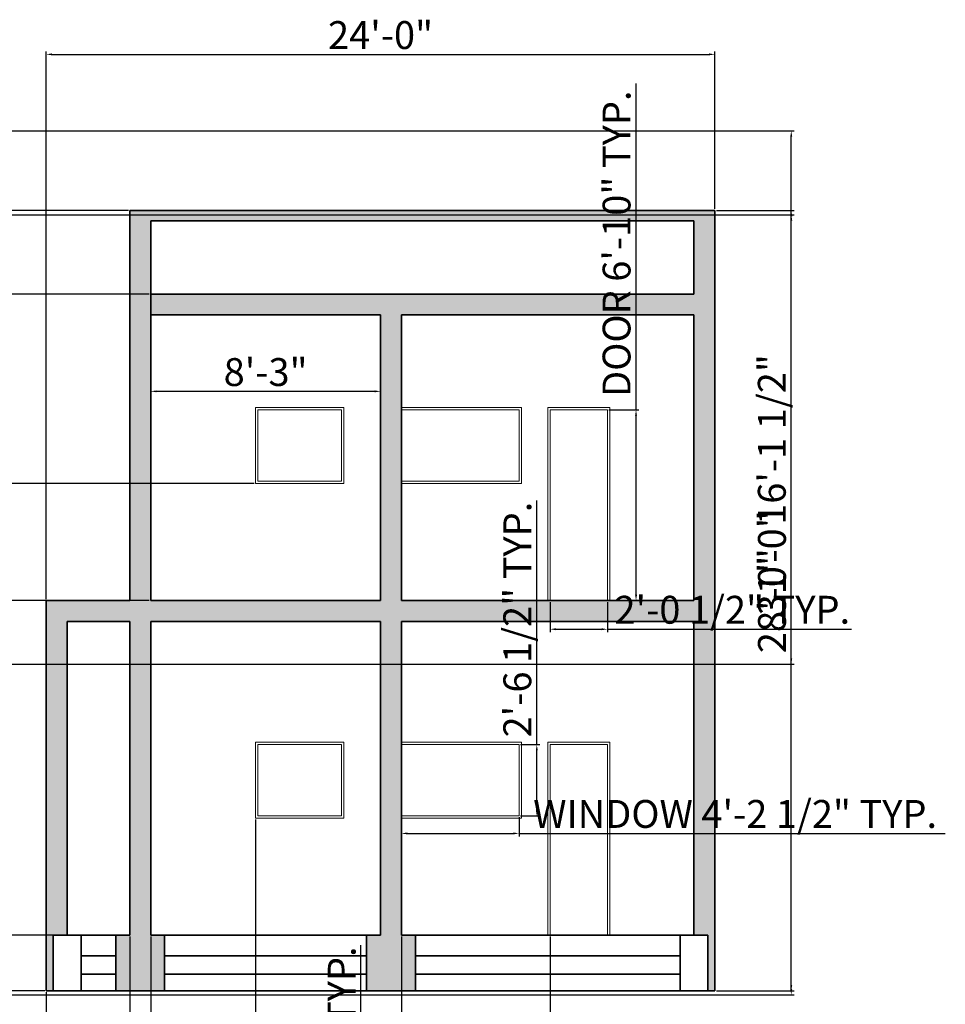
# Model space of a CAD drawing. Units: inches. Extents: x 2693 to 3501, y 1190 to 2292.
# Tile 4 of 4: x 3102 to 3501, y 1858 to 2282. Entities that reach past the tile are written whole.
import ezdxf

# ---------------------------------------------------------------- set-up
doc = ezdxf.new("R2010")
doc.units = ezdxf.units.IN
for name, color, linetype, lineweight in [('A-ANNO-DIMS', 2, 'Continuous', 18), ('A-DOOR', 3, 'Continuous', 18), ('A-GLAZ', 4, 'Continuous', 18), ('A-SECT', 7, 'Continuous', 35), ('A-SECT-PATT', 252, 'Continuous', 13)]:
    doc.layers.add(name, color=color, linetype=linetype, lineweight=lineweight)
doc.styles.get("Standard").update_dxf_attribs({"font": 'arial.ttf'})
doc.dimstyles.new('ISO-25', dxfattribs={"dimtxt": 12, "dimasz": 2.5, "dimexe": 1.25, "dimexo": 0.625, "dimtad": 1, "dimdec": 1, "dimlunit": 3, "dimtxsty": 'Standard', "dimcen": 2.5, "dimadec": 0, "dimazin": 0, "dimtfac": 1, "dimtdec": 1, "dimtmove": 0, "dimatfit": 3, "dimfxl": 1, "dimarcsym": 0})

# ---------------------------------------------------------------- blocks, each defined once
blk = doc.blocks.new('DOOR-SECT-FRAME')
blk.add_lwpolyline([(24.72, 0), (24.72, 82.12), (0, 82.12), (0, 0)])
blk = doc.blocks.new('WIN-SECT-FRAME-RETURN')
blk.add_lwpolyline([(0, 30.69), (50.69, 30.69), (50.69, 0), (0, 0)])
blk = doc.blocks.new('*D10')
at = {"layer": 'A-ANNO-DIMS', "color": 0, "lineweight": -2, "transparency": 16777216}
for p, q in [((3248.85, 1806.53), (3248.85, 1883.43)), ((3241.37, 1806.53), (3250.1, 1806.53)), ((3248.85, 1800.03), (3248.85, 1804.03)), ((3241.37, 1797.53), (3250.1, 1797.53))]:
    blk.add_line(p, q, dxfattribs=at)
at = {"layer": 'A-ANNO-DIMS', "color": 0, "transparency": 16777216}
for points in [[(3248.43, 1804.03), (3249.26, 1804.03), (3248.85, 1806.53)], [(3248.43, 1800.03), (3249.26, 1800.03), (3248.85, 1797.53)]]:
    blk.add_solid(points, dxfattribs=at)
at = {"layer": 'Defpoints', "color": 0, "transparency": 16777216}
for p in [(3240.75, 1806.53), (3248.85, 1806.53), (3240.75, 1797.53)]:
    blk.add_point(p, dxfattribs=at)
at = {"layer": 'A-ANNO-DIMS', "color": 0, "transparency": 16777216, "insert": (3242.09, 1846.23), "char_height": 12, "attachment_point": 5, "rotation": 90}
blk.add_mtext('0\'-9" TYP.', dxfattribs=at)
blk = doc.blocks.new('*D17')
at = {"layer": 'A-ANNO-DIMS', "color": 0, "lineweight": -2, "transparency": 16777216}
for p, q in [((3266.27, 1938.47), (3266.27, 1930.24)), ((3316.96, 1938.47), (3316.96, 1930.24)), ((3268.77, 1931.49), (3314.46, 1931.49)), ((3316.96, 1931.49), (3500.52, 1931.49))]:
    blk.add_line(p, q, dxfattribs=at)
at = {"layer": 'A-ANNO-DIMS', "color": 0, "transparency": 16777216}
for points in [[(3268.77, 1931.91), (3268.77, 1931.08), (3266.27, 1931.49)], [(3314.46, 1931.91), (3314.46, 1931.08), (3316.96, 1931.49)]]:
    blk.add_solid(points, dxfattribs=at)
at = {"layer": 'Defpoints', "color": 0, "transparency": 16777216}
for p in [(3266.27, 1939.1), (3316.96, 1939.1), (3316.96, 1931.49)]:
    blk.add_point(p, dxfattribs=at)
at = {"layer": 'A-ANNO-DIMS', "color": 0, "transparency": 16777216, "insert": (3409.99, 1938.33), "char_height": 12, "attachment_point": 5}
blk.add_mtext('WINDOW 4\'-2 1/2" TYP.', dxfattribs=at)
blk = doc.blocks.new('*D18')
at = {"layer": 'A-ANNO-DIMS', "color": 0, "lineweight": -2, "transparency": 16777216}
for p, q in [((3324.56, 1969.78), (3324.56, 2074.85)), ((3317.59, 1969.78), (3325.81, 1969.78)), ((3324.56, 1941.6), (3324.56, 1967.28)), ((3317.59, 1939.1), (3325.81, 1939.1))]:
    blk.add_line(p, q, dxfattribs=at)
at = {"layer": 'A-ANNO-DIMS', "color": 0, "transparency": 16777216}
for points in [[(3324.15, 1967.28), (3324.98, 1967.28), (3324.56, 1969.78)], [(3324.15, 1941.6), (3324.98, 1941.6), (3324.56, 1939.1)]]:
    blk.add_solid(points, dxfattribs=at)
at = {"layer": 'Defpoints', "color": 0, "transparency": 16777216}
for p in [(3316.96, 1969.78), (3324.56, 1969.78), (3316.96, 1939.1)]:
    blk.add_point(p, dxfattribs=at)
at = {"layer": 'A-ANNO-DIMS', "color": 0, "transparency": 16777216, "insert": (3317.73, 2023.56), "char_height": 12, "attachment_point": 5, "rotation": 90}
blk.add_mtext('2\'-6 1/2" TYP.', dxfattribs=at)
blk = doc.blocks.new('*D19')
at = {"layer": 'A-ANNO-DIMS', "color": 0, "lineweight": -2, "transparency": 16777216}
for p, q in [((3367.31, 2113.83), (3367.31, 2254.41)), ((3355.62, 2113.83), (3368.56, 2113.83)), ((3367.31, 2034.22), (3367.31, 2111.33)), ((3355.62, 2031.72), (3368.56, 2031.72))]:
    blk.add_line(p, q, dxfattribs=at)
at = {"layer": 'A-ANNO-DIMS', "color": 0, "transparency": 16777216}
for points in [[(3366.89, 2111.33), (3367.73, 2111.33), (3367.31, 2113.83)], [(3366.89, 2034.22), (3367.73, 2034.22), (3367.31, 2031.72)]]:
    blk.add_solid(points, dxfattribs=at)
at = {"layer": 'Defpoints', "color": 0, "transparency": 16777216}
for p in [(3354.99, 2113.83), (3367.31, 2113.83), (3354.99, 2031.72)]:
    blk.add_point(p, dxfattribs=at)
at = {"layer": 'A-ANNO-DIMS', "color": 0, "transparency": 16777216, "insert": (3360.48, 2185.37), "char_height": 12, "attachment_point": 5, "rotation": 90}
blk.add_mtext('DOOR 6\'-10" TYP.', dxfattribs=at)
blk = doc.blocks.new('*D20')
at = {"layer": 'A-ANNO-DIMS', "color": 0, "lineweight": -2, "transparency": 16777216}
for p, q in [((3330.27, 2031.09), (3330.27, 2018.15)), ((3354.99, 2031.09), (3354.99, 2018.15)), ((3332.77, 2019.4), (3352.49, 2019.4)), ((3354.99, 2019.4), (3460.05, 2019.4))]:
    blk.add_line(p, q, dxfattribs=at)
at = {"layer": 'A-ANNO-DIMS', "color": 0, "transparency": 16777216}
for points in [[(3332.77, 2019.82), (3332.77, 2018.98), (3330.27, 2019.4)], [(3352.49, 2019.82), (3352.49, 2018.98), (3354.99, 2019.4)]]:
    blk.add_solid(points, dxfattribs=at)
at = {"layer": 'Defpoints', "color": 0, "transparency": 16777216}
for p in [(3330.27, 2031.72), (3354.99, 2031.72), (3354.99, 2019.4)]:
    blk.add_point(p, dxfattribs=at)
at = {"layer": 'A-ANNO-DIMS', "color": 0, "transparency": 16777216, "insert": (3408.77, 2026.23), "char_height": 12, "attachment_point": 5}
blk.add_mtext('2\'-0 1/2" TYP.', dxfattribs=at)
blk = doc.blocks.new('*D45')
at = {"layer": 'A-ANNO-DIMS', "color": 0, "lineweight": -2, "transparency": 16777216}
for p, q in [((3005.39, 2197.86), (3435.42, 2197.86)), ((3434.17, 2006.84), (3434.17, 2195.36)), ((3005.39, 2004.34), (3435.42, 2004.34))]:
    blk.add_line(p, q, dxfattribs=at)
at = {"layer": 'A-ANNO-DIMS', "color": 0, "transparency": 16777216}
for points in [[(3433.76, 2195.36), (3434.59, 2195.36), (3434.17, 2197.86)], [(3433.76, 2006.84), (3434.59, 2006.84), (3434.17, 2004.34)]]:
    blk.add_solid(points, dxfattribs=at)
at = {"layer": 'Defpoints', "color": 0, "transparency": 16777216}
for p in [(3004.76, 2197.86), (3434.17, 2197.86), (3004.76, 2004.34)]:
    blk.add_point(p, dxfattribs=at)
at = {"layer": 'A-ANNO-DIMS', "color": 0, "transparency": 16777216, "insert": (3427.34, 2101.1), "char_height": 12, "attachment_point": 5, "rotation": 90}
blk.add_mtext('16\'-1 1/2"', dxfattribs=at)
blk = doc.blocks.new('*D47')
at = {"layer": 'A-ANNO-DIMS', "color": 0, "lineweight": -2, "transparency": 16777216}
for p, q in [((3039.3, 2233.99), (3435.42, 2233.99)), ((3434.17, 1864.49), (3434.17, 2231.49)), ((3039.3, 1861.99), (3435.42, 1861.99))]:
    blk.add_line(p, q, dxfattribs=at)
at = {"layer": 'A-ANNO-DIMS', "color": 0, "transparency": 16777216}
for points in [[(3433.76, 2231.49), (3434.59, 2231.49), (3434.17, 2233.99)], [(3433.76, 1864.49), (3434.59, 1864.49), (3434.17, 1861.99)]]:
    blk.add_solid(points, dxfattribs=at)
at = {"layer": 'Defpoints', "color": 0, "transparency": 16777216}
for p in [(3038.68, 2233.99), (3434.17, 2233.99), (3038.68, 1861.99)]:
    blk.add_point(p, dxfattribs=at)
at = {"layer": 'A-ANNO-DIMS', "color": 0, "transparency": 16777216, "insert": (3427.42, 2047.99), "char_height": 12, "attachment_point": 5, "rotation": 90}
blk.add_mtext('31\'-0"', dxfattribs=at)
blk = doc.blocks.new('*D48')
at = {"layer": 'A-ANNO-DIMS', "color": 0, "lineweight": -2, "transparency": 16777216}
for p, q in [((2717.78, 1887.72), (2717.78, 1923.57)), ((3115.65, 1887.72), (2716.53, 1887.72)), ((2717.78, 1866.22), (2717.78, 1885.22)), ((3112.65, 1863.72), (2716.53, 1863.72))]:
    blk.add_line(p, q, dxfattribs=at)
at = {"layer": 'A-ANNO-DIMS', "color": 0, "transparency": 16777216}
for points in [[(2717.36, 1885.22), (2718.19, 1885.22), (2717.78, 1887.72)], [(2717.36, 1866.22), (2718.19, 1866.22), (2717.78, 1863.72)]]:
    blk.add_solid(points, dxfattribs=at)
at = {"layer": 'Defpoints', "color": 0, "transparency": 16777216}
for p in [(2717.78, 1887.72), (3116.27, 1887.72), (3113.27, 1863.72)]:
    blk.add_point(p, dxfattribs=at)
at = {"layer": 'A-ANNO-DIMS', "color": 0, "transparency": 16777216, "insert": (2711.02, 1906.89), "char_height": 12, "attachment_point": 5, "rotation": 90}
blk.add_mtext('2\'-0"', dxfattribs=at)
blk = doc.blocks.new('*D49')
at = {"layer": 'A-ANNO-DIMS', "color": 0, "lineweight": -2, "transparency": 16777216}
for p, q in [((3112.65, 2031.72), (2716.53, 2031.72)), ((2717.78, 1890.22), (2717.78, 2029.22)), ((3121.65, 1887.72), (2716.53, 1887.72))]:
    blk.add_line(p, q, dxfattribs=at)
at = {"layer": 'A-ANNO-DIMS', "color": 0, "transparency": 16777216}
for points in [[(2717.36, 2029.22), (2718.19, 2029.22), (2717.78, 2031.72)], [(2717.36, 1890.22), (2718.19, 1890.22), (2717.78, 1887.72)]]:
    blk.add_solid(points, dxfattribs=at)
at = {"layer": 'Defpoints', "color": 0, "transparency": 16777216}
for p in [(2717.78, 2031.72), (3113.27, 2031.72), (3122.27, 1887.72)]:
    blk.add_point(p, dxfattribs=at)
at = {"layer": 'A-ANNO-DIMS', "color": 0, "transparency": 16777216, "insert": (2711.02, 1959.72), "char_height": 12, "attachment_point": 5, "rotation": 90}
blk.add_mtext('12\'-0"', dxfattribs=at)
blk = doc.blocks.new('*D50')
at = {"layer": 'A-ANNO-DIMS', "color": 0, "lineweight": -2, "transparency": 16777216}
for p, q in [((3157.65, 2163.72), (2716.53, 2163.72)), ((2717.78, 2034.22), (2717.78, 2161.22)), ((3112.65, 2031.72), (2716.53, 2031.72))]:
    blk.add_line(p, q, dxfattribs=at)
at = {"layer": 'A-ANNO-DIMS', "color": 0, "transparency": 16777216}
for points in [[(2717.36, 2161.22), (2718.19, 2161.22), (2717.78, 2163.72)], [(2717.36, 2034.22), (2718.19, 2034.22), (2717.78, 2031.72)]]:
    blk.add_solid(points, dxfattribs=at)
at = {"layer": 'Defpoints', "color": 0, "transparency": 16777216}
for p in [(2717.78, 2163.72), (3158.27, 2163.72), (3113.27, 2031.72)]:
    blk.add_point(p, dxfattribs=at)
at = {"layer": 'A-ANNO-DIMS', "color": 0, "transparency": 16777216, "insert": (2711.02, 2097.72), "char_height": 12, "attachment_point": 5, "rotation": 90}
blk.add_mtext('11\'-0"', dxfattribs=at)
blk = doc.blocks.new('*D51')
at = {"layer": 'A-ANNO-DIMS', "color": 0, "lineweight": -2, "transparency": 16777216}
for p, q in [((3148.65, 2199.72), (2716.53, 2199.72)), ((2717.78, 2166.22), (2717.78, 2197.22)), ((3157.65, 2163.72), (2716.53, 2163.72))]:
    blk.add_line(p, q, dxfattribs=at)
at = {"layer": 'A-ANNO-DIMS', "color": 0, "transparency": 16777216}
for points in [[(2717.36, 2197.22), (2718.19, 2197.22), (2717.78, 2199.72)], [(2717.36, 2166.22), (2718.19, 2166.22), (2717.78, 2163.72)]]:
    blk.add_solid(points, dxfattribs=at)
at = {"layer": 'Defpoints', "color": 0, "transparency": 16777216}
for p in [(2717.78, 2199.72), (3149.27, 2199.72), (3158.27, 2163.72)]:
    blk.add_point(p, dxfattribs=at)
at = {"layer": 'A-ANNO-DIMS', "color": 0, "transparency": 16777216, "insert": (2711.02, 2181.72), "char_height": 12, "attachment_point": 5, "rotation": 90}
blk.add_mtext('3\'-0"', dxfattribs=at)
blk = doc.blocks.new('*D52')
at = {"layer": 'A-ANNO-DIMS', "color": 0, "lineweight": -2, "transparency": 16777216}
for p, q in [((3149.27, 1887.09), (3149.27, 1804.29)), ((3113.27, 1863.09), (3113.27, 1804.29)), ((3146.77, 1805.54), (3115.77, 1805.54))]:
    blk.add_line(p, q, dxfattribs=at)
at = {"layer": 'A-ANNO-DIMS', "color": 0, "transparency": 16777216}
for points in [[(3115.77, 1805.95), (3115.77, 1805.12), (3113.27, 1805.54)], [(3146.77, 1805.95), (3146.77, 1805.12), (3149.27, 1805.54)]]:
    blk.add_solid(points, dxfattribs=at)
at = {"layer": 'Defpoints', "color": 0, "transparency": 16777216}
for p in [(3149.27, 1887.72), (3113.27, 1863.72), (3113.27, 1805.54)]:
    blk.add_point(p, dxfattribs=at)
at = {"layer": 'A-ANNO-DIMS', "color": 0, "transparency": 16777216, "insert": (3131.27, 1812.29), "char_height": 12, "attachment_point": 5}
blk.add_mtext('3\'-0"', dxfattribs=at)
blk = doc.blocks.new('*D53')
at = {"layer": 'A-ANNO-DIMS', "color": 0, "lineweight": -2, "transparency": 16777216}
for p, q in [((3158.27, 2154.09), (3158.27, 2120.57)), ((3257.27, 2154.09), (3257.27, 2120.57)), ((3254.77, 2121.82), (3160.77, 2121.82))]:
    blk.add_line(p, q, dxfattribs=at)
at = {"layer": 'A-ANNO-DIMS', "color": 0, "transparency": 16777216}
for points in [[(3160.77, 2122.23), (3160.77, 2121.4), (3158.27, 2121.82)], [(3254.77, 2122.23), (3254.77, 2121.4), (3257.27, 2121.82)]]:
    blk.add_solid(points, dxfattribs=at)
at = {"layer": 'Defpoints', "color": 0, "transparency": 16777216}
for p in [(3158.27, 2154.72), (3257.27, 2154.72), (3158.27, 2121.82)]:
    blk.add_point(p, dxfattribs=at)
at = {"layer": 'A-ANNO-DIMS', "color": 0, "transparency": 16777216, "insert": (3207.77, 2128.57), "char_height": 12, "attachment_point": 5}
blk.add_mtext('8\'-3"', dxfattribs=at)
blk = doc.blocks.new('*D54')
at = {"layer": 'A-ANNO-DIMS', "color": 0, "lineweight": -2, "transparency": 16777216}
for p, q in [((3203.45, 1937.47), (3203.45, 1804.29)), ((3158.27, 1887.09), (3158.27, 1804.29)), ((3160.77, 1805.54), (3200.95, 1805.54))]:
    blk.add_line(p, q, dxfattribs=at)
at = {"layer": 'A-ANNO-DIMS', "color": 0, "transparency": 16777216}
for points in [[(3160.77, 1805.95), (3160.77, 1805.12), (3158.27, 1805.54)], [(3200.95, 1805.95), (3200.95, 1805.12), (3203.45, 1805.54)]]:
    blk.add_solid(points, dxfattribs=at)
at = {"layer": 'Defpoints', "color": 0, "transparency": 16777216}
for p in [(3203.45, 1938.1), (3158.27, 1887.72), (3203.45, 1805.54)]:
    blk.add_point(p, dxfattribs=at)
at = {"layer": 'A-ANNO-DIMS', "color": 0, "transparency": 16777216, "insert": (3180.86, 1812.29), "char_height": 12, "attachment_point": 5}
blk.add_mtext('3\'-9"', dxfattribs=at)
blk = doc.blocks.new('*D55')
at = {"layer": 'A-ANNO-DIMS', "color": 0, "lineweight": -2, "transparency": 16777216}
for p, q in [((3266.27, 1887.09), (3266.27, 1804.29)), ((3330.27, 1887.09), (3330.27, 1804.29)), ((3268.77, 1805.54), (3327.77, 1805.54))]:
    blk.add_line(p, q, dxfattribs=at)
at = {"layer": 'A-ANNO-DIMS', "color": 0, "transparency": 16777216}
for points in [[(3268.77, 1805.95), (3268.77, 1805.12), (3266.27, 1805.54)], [(3327.77, 1805.95), (3327.77, 1805.12), (3330.27, 1805.54)]]:
    blk.add_solid(points, dxfattribs=at)
at = {"layer": 'Defpoints', "color": 0, "transparency": 16777216}
for p in [(3266.27, 1887.72), (3330.27, 1887.72), (3330.27, 1805.54)]:
    blk.add_point(p, dxfattribs=at)
at = {"layer": 'A-ANNO-DIMS', "color": 0, "transparency": 16777216, "insert": (3298.27, 1812.26), "char_height": 12, "attachment_point": 5}
blk.add_mtext('5\'-4"', dxfattribs=at)
blk = doc.blocks.new('*D56')
at = {"layer": 'A-ANNO-DIMS', "color": 0, "lineweight": -2, "transparency": 16777216}
for p, q in [((3202.82, 2082.15), (2716.53, 2082.15)), ((2717.78, 2079.65), (2717.78, 2034.22)), ((3157.65, 2031.72), (2716.53, 2031.72)), ((2717.78, 2031.72), (2717.78, 1967.62))]:
    blk.add_line(p, q, dxfattribs=at)
at = {"layer": 'A-ANNO-DIMS', "color": 0, "transparency": 16777216}
for points in [[(2717.36, 2079.65), (2718.19, 2079.65), (2717.78, 2082.15)], [(2717.36, 2034.22), (2718.19, 2034.22), (2717.78, 2031.72)]]:
    blk.add_solid(points, dxfattribs=at)
at = {"layer": 'Defpoints', "color": 0, "transparency": 16777216}
for p in [(3203.45, 2082.15), (2717.78, 2031.72), (3158.27, 2031.72)]:
    blk.add_point(p, dxfattribs=at)
at = {"layer": 'A-ANNO-DIMS', "color": 0, "transparency": 16777216, "insert": (2710.95, 1998.42), "char_height": 12, "attachment_point": 5, "rotation": 90}
blk.add_mtext('4\'-2 1/2"', dxfattribs=at)
blk = doc.blocks.new('*D57')
at = {"layer": 'A-ANNO-DIMS', "color": 0, "lineweight": -2, "transparency": 16777216}
for p, q in [((3113.27, 2032.34), (3113.27, 2268.14)), ((3401.27, 2200.34), (3401.27, 2268.14)), ((3115.77, 2266.89), (3398.77, 2266.89))]:
    blk.add_line(p, q, dxfattribs=at)
at = {"layer": 'A-ANNO-DIMS', "color": 0, "transparency": 16777216}
for points in [[(3115.77, 2267.31), (3115.77, 2266.48), (3113.27, 2266.89)], [(3398.77, 2267.31), (3398.77, 2266.48), (3401.27, 2266.89)]]:
    blk.add_solid(points, dxfattribs=at)
at = {"layer": 'Defpoints', "color": 0, "transparency": 16777216}
for p in [(3401.27, 2266.89), (3401.27, 2199.72), (3113.27, 2031.72)]:
    blk.add_point(p, dxfattribs=at)
at = {"layer": 'A-ANNO-DIMS', "color": 0, "transparency": 16777216, "insert": (3257.27, 2273.65), "char_height": 12, "attachment_point": 5}
blk.add_mtext('24\'-0"', dxfattribs=at)
blk = doc.blocks.new('*D58')
at = {"layer": 'A-ANNO-DIMS', "color": 0, "lineweight": -2, "transparency": 16777216}
for p, q in [((3401.9, 2199.72), (3435.42, 2199.72)), ((3434.17, 1866.22), (3434.17, 2197.22)), ((3401.9, 1863.72), (3435.42, 1863.72))]:
    blk.add_line(p, q, dxfattribs=at)
at = {"layer": 'A-ANNO-DIMS', "color": 0, "transparency": 16777216}
for points in [[(3433.76, 2197.22), (3434.59, 2197.22), (3434.17, 2199.72)], [(3433.76, 1866.22), (3434.59, 1866.22), (3434.17, 1863.72)]]:
    blk.add_solid(points, dxfattribs=at)
at = {"layer": 'Defpoints', "color": 0, "transparency": 16777216}
for p in [(3401.27, 2199.72), (3434.17, 2199.72), (3401.27, 1863.72)]:
    blk.add_point(p, dxfattribs=at)
at = {"layer": 'A-ANNO-DIMS', "color": 0, "transparency": 16777216, "insert": (3427.42, 2031.72), "char_height": 12, "attachment_point": 5, "rotation": 90}
blk.add_mtext('28\'-0"', dxfattribs=at)

msp = doc.modelspace()

# ---------------------------------------------------------------- hatches: boundary and pattern name
at = {"layer": 'A-SECT-PATT'}
h = msp.add_hatch(color=256, dxfattribs=at)
h.dxf.hatch_style = 1
h.paths.add_polyline_path([(3038.68, 2197.99), (3038.68, 2233.99), (2879.9, 2233.99), (2879.9, 2224.99), (3029.68, 2224.99), (3029.68, 2193.49), (3029.68, 2161.99), (3029.68, 2029.99), (3029.68, 1962.38), (3029.68, 1890.49), (2903.68, 1890.49), (2786.68, 1890.49), (2780.68, 1890.49), (2759.68, 1890.49), (2755.18, 1890.49), (2755.18, 2020.99), (2894.68, 2020.99), (2894.68, 2029.99), (2786.68, 2029.99), (2750.68, 2029.99), (2750.68, 1861.99), (3038.68, 1861.99), (3038.68, 1885.99)])
h.paths.add_polyline_path([(3029.68, 1885.99), (3029.68, 1866.49), (2755.18, 1866.49), (2755.18, 1885.99), (2759.68, 1885.99), (2765.68, 1885.99), (2786.68, 1885.99), (2903.68, 1885.99), (2909.68, 1885.99), (2912.68, 1885.99)], flags=16)
h.paths.add_polyline_path([(2903.68, 2152.99), (2903.68, 2224.99), (2894.68, 2224.99), (2894.68, 2197.99), (2894.43, 2197.99), (2786.68, 2197.99), (2778.76, 2197.99), (2778.76, 2193.49), (2786.68, 2193.49), (2786.68, 2029.99), (2795.68, 2029.99), (2795.68, 2152.99), (2894.68, 2152.99), (2894.68, 2029.99), (2894.68, 1971.38), (2894.68, 1962.38), (3029.68, 1962.38), (3029.68, 1971.38), (2903.68, 1971.38), (2903.68, 2029.99)], flags=17)
h.paths.add_polyline_path([(2894.68, 2161.99), (2795.68, 2161.99), (2795.68, 2193.49), (2894.68, 2193.49)], flags=16)
h.paths.add_polyline_path([(3401.27, 2199.72), (3149.27, 2199.72), (3149.27, 2031.72), (3113.27, 2031.72), (3113.27, 1863.72), (3116.27, 1863.72), (3116.27, 1887.72), (3122.27, 1887.72), (3122.27, 2022.72), (3149.27, 2022.72), (3149.27, 1887.72), (3143.27, 1887.72), (3143.27, 1863.72), (3164.27, 1863.72), (3164.27, 1887.72), (3158.27, 1887.72), (3158.27, 2022.72), (3257.27, 2022.72), (3257.27, 1887.72), (3251.27, 1887.72), (3251.27, 1863.72), (3272.27, 1863.72), (3272.27, 1887.72), (3266.27, 1887.72), (3266.27, 2022.72), (3392.27, 2022.72), (3392.27, 1887.72), (3398.27, 1887.72), (3398.27, 1863.72), (3401.27, 1863.72), (3401.27, 1887.72)])
h.paths.add_polyline_path([(3257.27, 2031.72), (3158.27, 2031.72), (3158.27, 2195.22), (3392.27, 2195.22), (3392.27, 2163.72), (3158.27, 2163.72), (3158.27, 2154.72), (3257.27, 2154.72)], flags=16)
h.paths.add_polyline_path([(3266.27, 2031.72), (3266.27, 2154.72), (3392.27, 2154.72), (3392.27, 2031.72)], flags=16)
h.paths.add_polyline_path([(3266.27, 2082.15), (3266.27, 2114.83), (3317.96, 2114.83), (3317.96, 2082.15)], flags=0)
h.paths.add_polyline_path([(3241.51, 2082.15), (3203.45, 2082.15), (3203.45, 2114.83), (3241.51, 2114.83)], flags=0)
h.paths.add_polyline_path([(3240.51, 2083.15), (3204.45, 2083.15), (3204.45, 2113.83), (3240.51, 2113.83)], flags=0)
h.paths.add_polyline_path([(3329.27, 2031.72), (3329.27, 2114.83), (3355.99, 2114.83), (3355.99, 2031.72)], flags=0)

# ---------------------------------------------------------------- linework, layer by layer
at = {"layer": 'A-DOOR'}
for points in [[(3329.27, 2031.72), (3355.99, 2031.72), (3355.99, 2114.83), (3329.27, 2114.83)], [(3329.27, 1887.72), (3355.99, 1887.72), (3355.99, 1970.83), (3329.27, 1970.83)]]:
    msp.add_lwpolyline(points, close=True, dxfattribs=at)
at = {"layer": 'A-GLAZ'}
for p, q in [((3203.45, 1970.78), (3203.45, 1938.1)), ((3241.51, 1970.78), (3203.45, 1970.78)), ((3240.51, 1969.78), (3204.45, 1969.78)), ((3204.45, 1969.78), (3204.45, 1939.1)), ((3240.51, 1969.78), (3240.51, 1939.1)), ((3241.51, 1970.78), (3241.51, 1938.1)), ((3241.51, 1938.1), (3203.45, 1938.1)), ((3240.51, 1939.1), (3204.45, 1939.1))]:
    msp.add_line(p, q, dxfattribs=at)
for points in [[(3203.45, 2114.83), (3241.51, 2114.83), (3241.51, 2082.15), (3203.45, 2082.15)], [(3204.45, 2113.83), (3240.51, 2113.83), (3240.51, 2083.15), (3204.45, 2083.15)], [(3266.27, 2114.83), (3317.96, 2114.83), (3317.96, 2082.15), (3266.27, 2082.15)], [(3266.27, 1970.78), (3317.96, 1970.78), (3317.96, 1938.1), (3266.27, 1938.1)]]:
    msp.add_lwpolyline(points, close=True, dxfattribs=at)
at = {"layer": 'A-SECT'}
for p, q in [((3149.27, 2199.72), (3401.27, 2199.72)), ((3149.27, 2031.72), (3149.27, 2199.72)), ((3401.27, 1887.72), (3401.27, 2199.72)), ((3158.27, 2195.22), (3392.27, 2195.22)), ((3158.27, 2031.72), (3158.27, 2195.22)), ((3392.27, 2163.72), (3392.27, 2195.22)), ((3149.27, 2154.72), (3149.27, 2163.72)), ((3158.27, 2163.72), (3392.27, 2163.72)), ((3158.27, 2154.72), (3257.27, 2154.72)), ((3257.27, 2154.72), (3257.27, 2031.72)), ((3266.27, 2031.72), (3266.27, 2154.72)), ((3266.27, 2154.72), (3392.27, 2154.72)), ((3392.27, 2031.72), (3392.27, 2154.72)), ((3113.27, 1863.72), (3113.27, 2031.72)), ((3113.27, 2031.72), (3149.27, 2031.72)), ((3158.27, 2031.72), (3257.27, 2031.72)), ((3266.27, 2031.72), (3392.27, 2031.72)), ((3122.27, 1887.72), (3122.27, 2022.72)), ((3122.27, 2022.72), (3149.27, 2022.72)), ((3149.27, 1887.72), (3149.27, 2022.72)), ((3158.27, 1887.72), (3158.27, 2022.72)), ((3158.27, 2022.72), (3257.27, 2022.72)), ((3257.27, 2022.72), (3257.27, 1887.72)), ((3266.27, 1887.72), (3266.27, 2022.72)), ((3266.27, 2022.72), (3392.27, 2022.72)), ((3392.27, 1887.72), (3392.27, 2022.72)), ((3122.27, 1887.72), (3116.27, 1887.72)), ((3116.27, 1887.72), (3116.27, 1863.72)), ((3122.27, 1887.72), (3149.27, 1887.72)), ((3122.27, 1887.72), (3128.27, 1887.72)), ((3128.27, 1887.72), (3122.27, 1887.72)), ((3128.27, 1887.72), (3128.27, 1863.72)), ((3128.27, 1863.72), (3128.27, 1887.72)), ((3149.27, 1887.72), (3143.27, 1887.72)), ((3143.27, 1887.72), (3143.27, 1863.72)), ((3158.27, 1887.72), (3257.27, 1887.72)), ((3158.27, 1887.72), (3164.27, 1887.72)), ((3164.27, 1887.72), (3164.27, 1863.72)), ((3257.27, 1887.72), (3251.27, 1887.72)), ((3251.27, 1887.72), (3251.27, 1863.72)), ((3266.27, 1887.72), (3392.27, 1887.72)), ((3266.27, 1887.72), (3275.27, 1887.72)), ((3266.27, 1887.72), (3272.27, 1887.72)), ((3272.27, 1887.72), (3272.27, 1863.72)), ((3392.27, 1887.72), (3386.27, 1887.72)), ((3386.27, 1887.72), (3386.27, 1863.72)), ((3392.27, 1887.72), (3398.27, 1887.72)), ((3398.27, 1887.72), (3392.27, 1887.72)), ((3398.27, 1887.72), (3398.27, 1863.72)), ((3401.27, 1863.72), (3401.27, 1887.72)), ((3128.27, 1878.8), (3143.27, 1878.8)), ((3164.27, 1878.8), (3251.27, 1878.8)), ((3272.27, 1878.8), (3386.27, 1878.8)), ((3386.27, 1878.8), (3386.27, 1870.97)), ((3143.27, 1870.97), (3128.27, 1870.97)), ((3251.27, 1870.97), (3164.27, 1870.97)), ((3386.27, 1870.97), (3272.27, 1870.97)), ((3113.27, 1863.72), (3401.27, 1863.72))]:
    msp.add_line(p, q, dxfattribs=at)

# ---------------------------------------------------------------- block references
at = {"layer": 'A-DOOR'}
for p in [(3330.27, 2031.72), (3330.27, 1887.72)]:
    msp.add_blockref('DOOR-SECT-FRAME', p, dxfattribs=at)
at = {"layer": 'A-GLAZ'}
for p in [(3266.27, 2083.15), (3266.27, 1939.1)]:
    msp.add_blockref('WIN-SECT-FRAME-RETURN', p, dxfattribs=at)

# ---------------------------------------------------------------- dimensions: what is measured, and where the dimension line sits
at = {"layer": 'A-ANNO-DIMS'}
for base, p1, p2, picture, middle in [((3401.27, 2266.89), (3113.27, 2031.72), (3401.27, 2199.72), '*D57', (3257.27, 2273.65)), ((3203.45, 1805.54), (3158.27, 1887.72), (3203.45, 1938.1), '*D54', (3180.86, 1812.29)), ((3113.27, 1805.54), (3149.27, 1887.72), (3113.27, 1863.72), '*D52', (3131.27, 1812.29)), ((3330.27, 1805.54), (3266.27, 1887.72), (3330.27, 1887.72), '*D55', (3298.27, 1812.26))]:
    dim = msp.add_linear_dim(base=base, p1=p1, p2=p2, dimstyle='ISO-25', override={"dimdec": 1, "dimlfac": 1, "dimrnd": 0, "dimzin": 1, "dimdsep": 46, "dimlunit": 4, "dimfrac": 2}, dxfattribs=at)
    dim.commit()
    dim.dimension.update_dxf_attribs({"geometry": picture, "text_midpoint": middle})
for base, p1, p2, text, picture, middle in [((3367.31, 2113.83), (3354.99, 2031.72), (3354.99, 2113.83), 'DOOR <> TYP.', '*D19', (3360.48, 2185.37)), ((3324.56, 1969.78), (3316.96, 1939.1), (3316.96, 1969.78), '<> TYP.', '*D18', (3317.73, 2023.56)), ((3248.85, 1806.53), (3240.75, 1797.53), (3240.75, 1806.53), '<> TYP.', '*D10', (3242.09, 1846.23))]:
    dim = msp.add_linear_dim(base=base, p1=p1, p2=p2, angle=90, text=text, dimstyle='ISO-25', override={"dimdec": 1, "dimlfac": 1, "dimrnd": 0, "dimzin": 1, "dimdsep": 46, "dimlunit": 4, "dimfrac": 2}, dxfattribs=at)
    dim.commit()
    dim.dimension.update_dxf_attribs({"geometry": picture, "text_midpoint": middle})
for base, p1, p2, angle, picture, middle in [((3434.17, 2233.99), (3038.68, 1861.99), (3038.68, 2233.99), 90, '*D47', (3427.42, 2047.99)), ((2717.78, 2199.72), (3158.27, 2163.72), (3149.27, 2199.72), 90, '*D51', (2711.02, 2181.72)), ((3434.17, 2197.86), (3004.76, 2004.34), (3004.76, 2197.86), 90, '*D45', (3427.34, 2101.1)), ((3434.17, 2199.72), (3401.27, 1863.72), (3401.27, 2199.72), 90, '*D58', (3427.42, 2031.72)), ((2717.78, 2163.72), (3113.27, 2031.72), (3158.27, 2163.72), 90, '*D50', (2711.02, 2097.72)), ((3158.27, 2121.82), (3257.27, 2154.72), (3158.27, 2154.72), 180, '*D53', (3207.77, 2128.57)), ((2717.78, 2031.72), (3203.45, 2082.15), (3158.27, 2031.72), 90, '*D56', (2710.95, 1998.42)), ((2717.78, 2031.72), (3122.27, 1887.72), (3113.27, 2031.72), 90, '*D49', (2711.02, 1959.72)), ((2717.78, 1887.72), (3113.27, 1863.72), (3116.27, 1887.72), 90, '*D48', (2711.02, 1906.89))]:
    dim = msp.add_linear_dim(base=base, p1=p1, p2=p2, angle=angle, dimstyle='ISO-25', override={"dimdec": 1, "dimlfac": 1, "dimrnd": 0, "dimzin": 1, "dimdsep": 46, "dimlunit": 4, "dimfrac": 2}, dxfattribs=at)
    dim.commit()
    dim.dimension.update_dxf_attribs({"geometry": picture, "text_midpoint": middle})
for base, p1, p2, text, picture, middle in [((3354.99, 2019.4), (3330.27, 2031.72), (3354.99, 2031.72), '<> TYP.', '*D20', (3408.77, 2026.23)), ((3316.96, 1931.49), (3266.27, 1939.1), (3316.96, 1939.1), 'WINDOW <> TYP.', '*D17', (3409.99, 1938.33))]:
    dim = msp.add_linear_dim(base=base, p1=p1, p2=p2, text=text, dimstyle='ISO-25', override={"dimdec": 1, "dimlfac": 1, "dimrnd": 0, "dimzin": 1, "dimdsep": 46, "dimlunit": 4, "dimfrac": 2}, dxfattribs=at)
    dim.commit()
    dim.dimension.update_dxf_attribs({"geometry": picture, "text_midpoint": middle})

doc.saveas('drawing.dxf')
